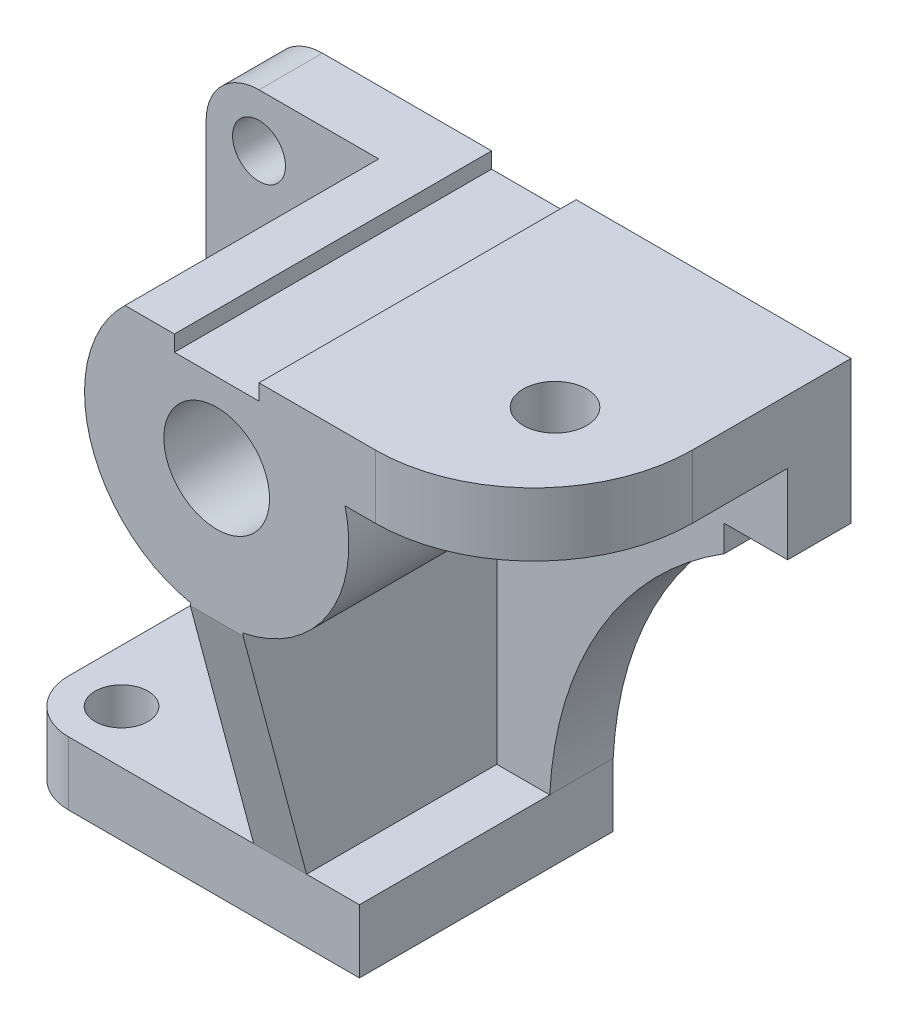
ISO-10303-21;
HEADER;
FILE_DESCRIPTION(('STEP AP214'),'2;1');
FILE_NAME('part.step','',(''),(''),'','','');
FILE_SCHEMA(('AUTOMOTIVE_DESIGN { 1 0 10303 214 1 1 1 1 }'));
ENDSEC;
DATA;
#1=APPLICATION_CONTEXT('core data for automotive mechanical design processes');
#2=APPLICATION_PROTOCOL_DEFINITION('international standard','automotive_design',2000,#1);
#3=PRODUCT_CONTEXT('',#1,'mechanical');
#4=PRODUCT('Part','Part','',(#3));
#5=PRODUCT_RELATED_PRODUCT_CATEGORY('part','',(#4));
#6=PRODUCT_DEFINITION_FORMATION('','',#4);
#7=PRODUCT_DEFINITION_CONTEXT('part definition',#1,'design');
#8=PRODUCT_DEFINITION('design','',#6,#7);
#9=PRODUCT_DEFINITION_SHAPE('','',#8);
#10=(LENGTH_UNIT() NAMED_UNIT(*) SI_UNIT(.MILLI.,.METRE.));
#11=(NAMED_UNIT(*) PLANE_ANGLE_UNIT() SI_UNIT($,.RADIAN.));
#12=(NAMED_UNIT(*) SI_UNIT($,.STERADIAN.) SOLID_ANGLE_UNIT());
#13=UNCERTAINTY_MEASURE_WITH_UNIT(LENGTH_MEASURE(1.E-05),#10,'distance_accuracy_value','');
#14=(GEOMETRIC_REPRESENTATION_CONTEXT(3) GLOBAL_UNCERTAINTY_ASSIGNED_CONTEXT((#13)) GLOBAL_UNIT_ASSIGNED_CONTEXT((#10,
#11,#12)) REPRESENTATION_CONTEXT('',''));
#15=CARTESIAN_POINT('',(0.,0.,0.));
#16=DIRECTION('',(0.,0.,1.));
#17=DIRECTION('',(1.,0.,0.));
#18=AXIS2_PLACEMENT_3D('',#15,#16,#17);
#19=CARTESIAN_POINT('',(102.413647614437,8.52410051292082,-12.));
#20=DIRECTION('',(0.,0.,1.));
#21=DIRECTION('',(1.,0.,0.));
#22=AXIS2_PLACEMENT_3D('',#19,#20,#21);
#23=PLANE('',#22);
#24=CARTESIAN_POINT('',(-22.5,90.,-12.));
#25=DIRECTION('',(0.,0.,1.));
#26=DIRECTION('',(1.,0.,0.));
#27=AXIS2_PLACEMENT_3D('',#24,#25,#26);
#28=CIRCLE('',#27,5.);
#29=CARTESIAN_POINT('',(-17.5,90.,-12.));
#30=VERTEX_POINT('',#29);
#31=EDGE_CURVE('E776',#30,#30,#28,.T.);
#32=ORIENTED_EDGE('',*,*,#31,.F.);
#33=EDGE_LOOP('',(#32));
#34=FACE_BOUND('',#33,.T.);
#35=DIRECTION('',(-1.,0.,0.));
#36=VECTOR('',#35,1.);
#37=CARTESIAN_POINT('',(32.5,12.,-12.));
#38=LINE('',#37,#36);
#39=CARTESIAN_POINT('',(12.5,12.,-12.));
#40=VERTEX_POINT('',#39);
#41=CARTESIAN_POINT('',(-32.5,12.,-12.));
#42=VERTEX_POINT('',#41);
#43=EDGE_CURVE('E300',#40,#42,#38,.T.);
#44=ORIENTED_EDGE('',*,*,#43,.F.);
#45=DIRECTION('',(0.,1.,0.));
#46=VECTOR('',#45,1.);
#47=CARTESIAN_POINT('',(12.5,8.52410051292082,-12.));
#48=LINE('',#47,#46);
#49=CARTESIAN_POINT('',(12.5,57.5051025721682,-12.));
#50=VERTEX_POINT('',#49);
#51=EDGE_CURVE('E232',#40,#50,#48,.T.);
#52=ORIENTED_EDGE('',*,*,#51,.T.);
#53=CARTESIAN_POINT('',(17.5,82.,-12.));
#54=DIRECTION('',(0.,0.,1.));
#55=DIRECTION('',(1.,0.,0.));
#56=AXIS2_PLACEMENT_3D('',#53,#54,#55);
#57=CIRCLE('',#56,25.);
#58=CARTESIAN_POINT('',(0.15064842710252,100.,-12.));
#59=VERTEX_POINT('',#58);
#60=EDGE_CURVE('E289',#59,#50,#57,.T.);
#61=ORIENTED_EDGE('',*,*,#60,.F.);
#62=DIRECTION('',(1.,0.,0.));
#63=VECTOR('',#62,1.);
#64=CARTESIAN_POINT('',(-32.5,100.,-12.));
#65=LINE('',#64,#63);
#66=CARTESIAN_POINT('',(-22.5,100.,-12.));
#67=VERTEX_POINT('',#66);
#68=EDGE_CURVE('E297',#67,#59,#65,.T.);
#69=ORIENTED_EDGE('',*,*,#68,.F.);
#70=CARTESIAN_POINT('',(-22.5,90.,-12.));
#71=DIRECTION('',(0.,0.,1.));
#72=DIRECTION('',(1.,0.,0.));
#73=AXIS2_PLACEMENT_3D('',#70,#71,#72);
#74=CIRCLE('',#73,10.);
#75=CARTESIAN_POINT('',(-32.5,90.,-12.));
#76=VERTEX_POINT('',#75);
#77=EDGE_CURVE('E381',#67,#76,#74,.T.);
#78=ORIENTED_EDGE('',*,*,#77,.T.);
#79=DIRECTION('',(0.,1.,0.));
#80=VECTOR('',#79,1.);
#81=CARTESIAN_POINT('',(-32.5,12.,-12.));
#82=LINE('',#81,#80);
#83=EDGE_CURVE('E298',#42,#76,#82,.T.);
#84=ORIENTED_EDGE('',*,*,#83,.F.);
#85=EDGE_LOOP('',(#44,#52,#61,#69,#78,#84));
#86=FACE_BOUND('',#85,.T.);
#87=ADVANCED_FACE('F43',(#34,#86),#23,.T.);
#88=CARTESIAN_POINT('',(0.,12.,0.));
#89=DIRECTION('',(0.,-1.,0.));
#90=DIRECTION('',(0.,0.,-1.));
#91=AXIS2_PLACEMENT_3D('',#88,#89,#90);
#92=PLANE('',#91);
#93=CARTESIAN_POINT('',(-22.5,12.,14.));
#94=DIRECTION('',(0.,1.,0.));
#95=DIRECTION('',(0.,0.,1.));
#96=AXIS2_PLACEMENT_3D('',#93,#94,#95);
#97=CIRCLE('',#96,5.);
#98=CARTESIAN_POINT('',(-22.5,12.,19.));
#99=VERTEX_POINT('',#98);
#100=EDGE_CURVE('E783',#99,#99,#97,.T.);
#101=ORIENTED_EDGE('',*,*,#100,.F.);
#102=EDGE_LOOP('',(#101));
#103=FACE_BOUND('',#102,.T.);
#104=DIRECTION('',(0.,0.,1.));
#105=VECTOR('',#104,1.);
#106=CARTESIAN_POINT('',(12.5,12.,0.));
#107=LINE('',#106,#105);
#108=CARTESIAN_POINT('',(12.5,12.,24.));
#109=VERTEX_POINT('',#108);
#110=EDGE_CURVE('E238',#40,#109,#107,.T.);
#111=ORIENTED_EDGE('',*,*,#110,.F.);
#112=ORIENTED_EDGE('',*,*,#43,.T.);
#113=DIRECTION('',(0.,0.,1.));
#114=VECTOR('',#113,1.);
#115=CARTESIAN_POINT('',(-32.5,12.,24.));
#116=LINE('',#115,#114);
#117=CARTESIAN_POINT('',(-32.5,12.,14.));
#118=VERTEX_POINT('',#117);
#119=EDGE_CURVE('E344',#42,#118,#116,.T.);
#120=ORIENTED_EDGE('',*,*,#119,.T.);
#121=CARTESIAN_POINT('',(-22.5,12.,14.));
#122=DIRECTION('',(0.,-1.,0.));
#123=DIRECTION('',(0.,0.,-1.));
#124=AXIS2_PLACEMENT_3D('',#121,#122,#123);
#125=CIRCLE('',#124,10.);
#126=CARTESIAN_POINT('',(-22.5,12.,24.));
#127=VERTEX_POINT('',#126);
#128=EDGE_CURVE('E374',#118,#127,#125,.F.);
#129=ORIENTED_EDGE('',*,*,#128,.T.);
#130=DIRECTION('',(1.,0.,0.));
#131=VECTOR('',#130,1.);
#132=CARTESIAN_POINT('',(-32.5,12.,24.));
#133=LINE('',#132,#131);
#134=EDGE_CURVE('E350',#127,#109,#133,.T.);
#135=ORIENTED_EDGE('',*,*,#134,.T.);
#136=EDGE_LOOP('',(#111,#112,#120,#129,#135));
#137=FACE_BOUND('',#136,.T.);
#138=ADVANCED_FACE('F472',(#103,#137),#92,.F.);
#139=CARTESIAN_POINT('',(17.5,82.,36.));
#140=DIRECTION('',(0.,0.,-1.));
#141=DIRECTION('',(-1.,0.,0.));
#142=AXIS2_PLACEMENT_3D('',#139,#140,#141);
#143=CYLINDRICAL_SURFACE('',#142,25.);
#144=DIRECTION('',(0.,0.,-1.));
#145=VECTOR('',#144,1.);
#146=CARTESIAN_POINT('',(12.5,57.5051025721682,36.));
#147=LINE('',#146,#145);
#148=CARTESIAN_POINT('',(12.5,57.5051025721682,36.));
#149=VERTEX_POINT('',#148);
#150=EDGE_CURVE('E214',#149,#50,#147,.T.);
#151=ORIENTED_EDGE('',*,*,#150,.F.);
#152=CARTESIAN_POINT('',(17.5,82.,36.));
#153=DIRECTION('',(0.,0.,1.));
#154=DIRECTION('',(1.,0.,0.));
#155=AXIS2_PLACEMENT_3D('',#152,#153,#154);
#156=CIRCLE('',#155,25.);
#157=CARTESIAN_POINT('',(0.15064842710252,100.,36.));
#158=VERTEX_POINT('',#157);
#159=EDGE_CURVE('E282',#158,#149,#156,.T.);
#160=ORIENTED_EDGE('',*,*,#159,.F.);
#161=DIRECTION('',(0.,0.,-1.));
#162=VECTOR('',#161,1.);
#163=CARTESIAN_POINT('',(0.15064842710252,100.,36.));
#164=LINE('',#163,#162);
#165=EDGE_CURVE('E287',#158,#59,#164,.T.);
#166=ORIENTED_EDGE('',*,*,#165,.T.);
#167=ORIENTED_EDGE('',*,*,#60,.T.);
#168=EDGE_LOOP('',(#151,#160,#166,#167));
#169=FACE_BOUND('',#168,.T.);
#170=ADVANCED_FACE('F458',(#169),#143,.T.);
#171=CARTESIAN_POINT('',(-32.5,100.,-12.));
#172=DIRECTION('',(0.,1.,0.));
#173=DIRECTION('',(-1.,0.,0.));
#174=AXIS2_PLACEMENT_3D('',#171,#172,#173);
#175=PLANE('',#174);
#176=CARTESIAN_POINT('',(57.5,100.,12.));
#177=DIRECTION('',(0.,1.,0.));
#178=DIRECTION('',(-1.,0.,0.));
#179=AXIS2_PLACEMENT_3D('',#176,#177,#178);
#180=CIRCLE('',#179,5.99999999999999);
#181=CARTESIAN_POINT('',(51.5,100.,12.));
#182=VERTEX_POINT('',#181);
#183=EDGE_CURVE('E771',#182,#182,#180,.T.);
#184=ORIENTED_EDGE('',*,*,#183,.F.);
#185=EDGE_LOOP('',(#184));
#186=FACE_BOUND('',#185,.T.);
#187=DIRECTION('',(-1.,0.,0.));
#188=VECTOR('',#187,1.);
#189=CARTESIAN_POINT('',(0.15064842710252,100.,36.));
#190=LINE('',#189,#188);
#191=CARTESIAN_POINT('',(47.5,100.,36.));
#192=VERTEX_POINT('',#191);
#193=CARTESIAN_POINT('',(25.5,100.,36.));
#194=VERTEX_POINT('',#193);
#195=EDGE_CURVE('E283',#192,#194,#190,.T.);
#196=ORIENTED_EDGE('',*,*,#195,.F.);
#197=CARTESIAN_POINT('',(47.5,100.,6.));
#198=DIRECTION('',(0.,1.,0.));
#199=DIRECTION('',(-1.,0.,0.));
#200=AXIS2_PLACEMENT_3D('',#197,#198,#199);
#201=CIRCLE('',#200,30.);
#202=CARTESIAN_POINT('',(77.5,100.,6.));
#203=VERTEX_POINT('',#202);
#204=EDGE_CURVE('E392',#192,#203,#201,.T.);
#205=ORIENTED_EDGE('',*,*,#204,.T.);
#206=DIRECTION('',(0.,0.,-1.));
#207=VECTOR('',#206,1.);
#208=CARTESIAN_POINT('',(77.5,100.,-12.));
#209=LINE('',#208,#207);
#210=CARTESIAN_POINT('',(77.5,100.,-24.));
#211=VERTEX_POINT('',#210);
#212=EDGE_CURVE('E313',#203,#211,#209,.T.);
#213=ORIENTED_EDGE('',*,*,#212,.T.);
#214=DIRECTION('',(1.,0.,0.));
#215=VECTOR('',#214,1.);
#216=CARTESIAN_POINT('',(-32.5,100.,-24.));
#217=LINE('',#216,#215);
#218=CARTESIAN_POINT('',(25.5,100.,-24.));
#219=VERTEX_POINT('',#218);
#220=EDGE_CURVE('E292',#219,#211,#217,.T.);
#221=ORIENTED_EDGE('',*,*,#220,.F.);
#222=DIRECTION('',(0.,0.,-1.));
#223=VECTOR('',#222,1.);
#224=CARTESIAN_POINT('',(25.5,100.,-12.));
#225=LINE('',#224,#223);
#226=EDGE_CURVE('E279',#194,#219,#225,.T.);
#227=ORIENTED_EDGE('',*,*,#226,.F.);
#228=EDGE_LOOP('',(#196,#205,#213,#221,#227));
#229=FACE_BOUND('',#228,.T.);
#230=ADVANCED_FACE('F391',(#186,#229),#175,.T.);
#231=DIRECTION('',(0.,1.,0.));
#232=VECTOR('',#231,1.);
#233=CARTESIAN_POINT('',(22.5,8.52410051292082,-12.));
#234=LINE('',#233,#232);
#235=CARTESIAN_POINT('',(22.5,12.,-12.));
#236=VERTEX_POINT('',#235);
#237=CARTESIAN_POINT('',(22.5,57.5051025721682,-12.));
#238=VERTEX_POINT('',#237);
#239=EDGE_CURVE('E241',#236,#238,#234,.T.);
#240=ORIENTED_EDGE('',*,*,#239,.F.);
#241=CARTESIAN_POINT('',(32.5,12.,-12.));
#242=VERTEX_POINT('',#241);
#243=EDGE_CURVE('E291',#242,#236,#38,.T.);
#244=ORIENTED_EDGE('',*,*,#243,.F.);
#245=CARTESIAN_POINT('',(102.413647614437,8.52410051292082,-12.));
#246=DIRECTION('',(0.,0.,1.));
#247=DIRECTION('',(1.,0.,0.));
#248=AXIS2_PLACEMENT_3D('',#245,#246,#247);
#249=CIRCLE('',#248,70.);
#250=CARTESIAN_POINT('',(65.5,68.,-12.));
#251=VERTEX_POINT('',#250);
#252=EDGE_CURVE('E311',#251,#242,#249,.T.);
#253=ORIENTED_EDGE('',*,*,#252,.F.);
#254=DIRECTION('',(0.,-1.,0.));
#255=VECTOR('',#254,1.);
#256=CARTESIAN_POINT('',(65.5,73.,-12.));
#257=LINE('',#256,#255);
#258=CARTESIAN_POINT('',(65.5,73.,-12.));
#259=VERTEX_POINT('',#258);
#260=EDGE_CURVE('E308',#259,#251,#257,.T.);
#261=ORIENTED_EDGE('',*,*,#260,.F.);
#262=DIRECTION('',(-1.,0.,0.));
#263=VECTOR('',#262,1.);
#264=CARTESIAN_POINT('',(77.5,73.,-12.));
#265=LINE('',#264,#263);
#266=CARTESIAN_POINT('',(77.5,73.,-12.));
#267=VERTEX_POINT('',#266);
#268=EDGE_CURVE('E304',#267,#259,#265,.T.);
#269=ORIENTED_EDGE('',*,*,#268,.F.);
#270=DIRECTION('',(0.,-1.,0.));
#271=VECTOR('',#270,1.);
#272=CARTESIAN_POINT('',(77.5,100.,-12.));
#273=LINE('',#272,#271);
#274=CARTESIAN_POINT('',(77.5,88.,-12.));
#275=VERTEX_POINT('',#274);
#276=EDGE_CURVE('E303',#275,#267,#273,.T.);
#277=ORIENTED_EDGE('',*,*,#276,.F.);
#278=DIRECTION('',(1.,0.,0.));
#279=VECTOR('',#278,1.);
#280=CARTESIAN_POINT('',(102.413647614437,88.,-12.));
#281=LINE('',#280,#279);
#282=CARTESIAN_POINT('',(41.7693221990232,88.,-12.));
#283=VERTEX_POINT('',#282);
#284=EDGE_CURVE('E251',#283,#275,#281,.T.);
#285=ORIENTED_EDGE('',*,*,#284,.F.);
#286=EDGE_CURVE('E278',#238,#283,#57,.T.);
#287=ORIENTED_EDGE('',*,*,#286,.F.);
#288=EDGE_LOOP('',(#240,#244,#253,#261,#269,#277,#285,#287));
#289=FACE_BOUND('',#288,.T.);
#290=ADVANCED_FACE('F411',(#289),#23,.T.);
#291=CARTESIAN_POINT('',(32.5,12.,24.));
#292=DIRECTION('',(-1.,0.,0.));
#293=DIRECTION('',(0.,0.,1.));
#294=AXIS2_PLACEMENT_3D('',#291,#292,#293);
#295=PLANE('',#294);
#296=DIRECTION('',(0.,0.,-1.));
#297=VECTOR('',#296,1.);
#298=CARTESIAN_POINT('',(32.5,0.,24.));
#299=LINE('',#298,#297);
#300=CARTESIAN_POINT('',(32.5,0.,24.));
#301=VERTEX_POINT('',#300);
#302=CARTESIAN_POINT('',(32.5,0.,-24.));
#303=VERTEX_POINT('',#302);
#304=EDGE_CURVE('E331',#301,#303,#299,.T.);
#305=ORIENTED_EDGE('',*,*,#304,.T.);
#306=DIRECTION('',(0.,-1.,0.));
#307=VECTOR('',#306,1.);
#308=CARTESIAN_POINT('',(32.5,12.,-24.));
#309=LINE('',#308,#307);
#310=CARTESIAN_POINT('',(32.5,12.,-24.));
#311=VERTEX_POINT('',#310);
#312=EDGE_CURVE('E364',#311,#303,#309,.T.);
#313=ORIENTED_EDGE('',*,*,#312,.F.);
#314=DIRECTION('',(0.,0.,-1.));
#315=VECTOR('',#314,1.);
#316=CARTESIAN_POINT('',(32.5,12.,-12.));
#317=LINE('',#316,#315);
#318=EDGE_CURVE('E326',#242,#311,#317,.T.);
#319=ORIENTED_EDGE('',*,*,#318,.F.);
#320=DIRECTION('',(0.,0.,-1.));
#321=VECTOR('',#320,1.);
#322=CARTESIAN_POINT('',(32.5,12.,24.));
#323=LINE('',#322,#321);
#324=CARTESIAN_POINT('',(32.5,12.,24.));
#325=VERTEX_POINT('',#324);
#326=EDGE_CURVE('E338',#325,#242,#323,.T.);
#327=ORIENTED_EDGE('',*,*,#326,.F.);
#328=DIRECTION('',(0.,-1.,0.));
#329=VECTOR('',#328,1.);
#330=CARTESIAN_POINT('',(32.5,12.,24.));
#331=LINE('',#330,#329);
#332=EDGE_CURVE('E348',#325,#301,#331,.T.);
#333=ORIENTED_EDGE('',*,*,#332,.T.);
#334=EDGE_LOOP('',(#305,#313,#319,#327,#333));
#335=FACE_BOUND('',#334,.T.);
#336=ADVANCED_FACE('F482',(#335),#295,.F.);
#337=CARTESIAN_POINT('',(-32.5,12.,-24.));
#338=DIRECTION('',(0.,0.,1.));
#339=DIRECTION('',(1.,0.,0.));
#340=AXIS2_PLACEMENT_3D('',#337,#338,#339);
#341=PLANE('',#340);
#342=CARTESIAN_POINT('',(17.5,82.,-24.));
#343=DIRECTION('',(0.,0.,1.));
#344=DIRECTION('',(1.,0.,0.));
#345=AXIS2_PLACEMENT_3D('',#342,#343,#344);
#346=CIRCLE('',#345,10.);
#347=CARTESIAN_POINT('',(27.5,82.,-24.));
#348=VERTEX_POINT('',#347);
#349=EDGE_CURVE('E789',#348,#348,#346,.F.);
#350=ORIENTED_EDGE('',*,*,#349,.F.);
#351=EDGE_LOOP('',(#350));
#352=FACE_BOUND('',#351,.T.);
#353=CARTESIAN_POINT('',(-22.5,90.,-24.));
#354=DIRECTION('',(0.,0.,1.));
#355=DIRECTION('',(1.,0.,0.));
#356=AXIS2_PLACEMENT_3D('',#353,#354,#355);
#357=CIRCLE('',#356,5.);
#358=CARTESIAN_POINT('',(-17.5,90.,-24.));
#359=VERTEX_POINT('',#358);
#360=EDGE_CURVE('E780',#359,#359,#357,.T.);
#361=ORIENTED_EDGE('',*,*,#360,.T.);
#362=EDGE_LOOP('',(#361));
#363=FACE_BOUND('',#362,.T.);
#364=DIRECTION('',(-1.,0.,0.));
#365=VECTOR('',#364,1.);
#366=CARTESIAN_POINT('',(-32.5,0.,-24.));
#367=LINE('',#366,#365);
#368=CARTESIAN_POINT('',(-32.5,0.,-24.));
#369=VERTEX_POINT('',#368);
#370=EDGE_CURVE('E354',#303,#369,#367,.T.);
#371=ORIENTED_EDGE('',*,*,#370,.T.);
#372=DIRECTION('',(0.,-1.,0.));
#373=VECTOR('',#372,1.);
#374=CARTESIAN_POINT('',(-32.5,12.,-24.));
#375=LINE('',#374,#373);
#376=CARTESIAN_POINT('',(-32.5,90.,-24.));
#377=VERTEX_POINT('',#376);
#378=EDGE_CURVE('E363',#377,#369,#375,.T.);
#379=ORIENTED_EDGE('',*,*,#378,.F.);
#380=CARTESIAN_POINT('',(-22.5,90.,-24.));
#381=DIRECTION('',(0.,0.,1.));
#382=DIRECTION('',(1.,0.,0.));
#383=AXIS2_PLACEMENT_3D('',#380,#381,#382);
#384=CIRCLE('',#383,10.);
#385=CARTESIAN_POINT('',(-22.5,100.,-24.));
#386=VERTEX_POINT('',#385);
#387=EDGE_CURVE('E379',#377,#386,#384,.F.);
#388=ORIENTED_EDGE('',*,*,#387,.T.);
#389=CARTESIAN_POINT('',(9.50000000000002,100.,-24.));
#390=VERTEX_POINT('',#389);
#391=EDGE_CURVE('E314',#386,#390,#217,.T.);
#392=ORIENTED_EDGE('',*,*,#391,.T.);
#393=DIRECTION('',(0.,-1.,0.));
#394=VECTOR('',#393,1.);
#395=CARTESIAN_POINT('',(9.50000000000002,97.,-24.));
#396=LINE('',#395,#394);
#397=CARTESIAN_POINT('',(9.50000000000002,97.,-24.));
#398=VERTEX_POINT('',#397);
#399=EDGE_CURVE('E262',#390,#398,#396,.T.);
#400=ORIENTED_EDGE('',*,*,#399,.T.);
#401=DIRECTION('',(1.,0.,0.));
#402=VECTOR('',#401,1.);
#403=CARTESIAN_POINT('',(9.50000000000002,97.,-24.));
#404=LINE('',#403,#402);
#405=CARTESIAN_POINT('',(25.5,97.,-24.));
#406=VERTEX_POINT('',#405);
#407=EDGE_CURVE('E263',#398,#406,#404,.T.);
#408=ORIENTED_EDGE('',*,*,#407,.T.);
#409=DIRECTION('',(0.,1.,0.));
#410=VECTOR('',#409,1.);
#411=CARTESIAN_POINT('',(25.5,97.,-24.));
#412=LINE('',#411,#410);
#413=EDGE_CURVE('E259',#406,#219,#412,.T.);
#414=ORIENTED_EDGE('',*,*,#413,.T.);
#415=ORIENTED_EDGE('',*,*,#220,.T.);
#416=DIRECTION('',(0.,-1.,0.));
#417=VECTOR('',#416,1.);
#418=CARTESIAN_POINT('',(77.5,100.,-24.));
#419=LINE('',#418,#417);
#420=CARTESIAN_POINT('',(77.5,73.,-24.));
#421=VERTEX_POINT('',#420);
#422=EDGE_CURVE('E319',#211,#421,#419,.T.);
#423=ORIENTED_EDGE('',*,*,#422,.T.);
#424=DIRECTION('',(-1.,0.,0.));
#425=VECTOR('',#424,1.);
#426=CARTESIAN_POINT('',(77.5,73.,-24.));
#427=LINE('',#426,#425);
#428=CARTESIAN_POINT('',(65.5,73.,-24.));
#429=VERTEX_POINT('',#428);
#430=EDGE_CURVE('E318',#421,#429,#427,.T.);
#431=ORIENTED_EDGE('',*,*,#430,.T.);
#432=DIRECTION('',(0.,-1.,0.));
#433=VECTOR('',#432,1.);
#434=CARTESIAN_POINT('',(65.5,73.,-24.));
#435=LINE('',#434,#433);
#436=CARTESIAN_POINT('',(65.5,68.,-24.));
#437=VERTEX_POINT('',#436);
#438=EDGE_CURVE('E324',#429,#437,#435,.T.);
#439=ORIENTED_EDGE('',*,*,#438,.T.);
#440=CARTESIAN_POINT('',(102.413647614437,8.52410051292082,-24.));
#441=DIRECTION('',(0.,0.,1.));
#442=DIRECTION('',(1.,0.,0.));
#443=AXIS2_PLACEMENT_3D('',#440,#441,#442);
#444=CIRCLE('',#443,70.);
#445=EDGE_CURVE('E327',#437,#311,#444,.T.);
#446=ORIENTED_EDGE('',*,*,#445,.T.);
#447=ORIENTED_EDGE('',*,*,#312,.T.);
#448=EDGE_LOOP('',(#371,#379,#388,#392,#400,#408,#414,#415,#423,#431,#439,#446,#447));
#449=FACE_BOUND('',#448,.T.);
#450=ADVANCED_FACE('F421',(#352,#363,#449),#341,.F.);
#451=CARTESIAN_POINT('',(-32.5,12.,24.));
#452=DIRECTION('',(1.,0.,0.));
#453=DIRECTION('',(0.,0.,-1.));
#454=AXIS2_PLACEMENT_3D('',#451,#452,#453);
#455=PLANE('',#454);
#456=ORIENTED_EDGE('',*,*,#83,.T.);
#457=DIRECTION('',(0.,0.,-1.));
#458=VECTOR('',#457,1.);
#459=CARTESIAN_POINT('',(-32.5,90.,-24.));
#460=LINE('',#459,#458);
#461=EDGE_CURVE('E380',#76,#377,#460,.T.);
#462=ORIENTED_EDGE('',*,*,#461,.T.);
#463=ORIENTED_EDGE('',*,*,#378,.T.);
#464=DIRECTION('',(0.,0.,1.));
#465=VECTOR('',#464,1.);
#466=CARTESIAN_POINT('',(-32.5,0.,24.));
#467=LINE('',#466,#465);
#468=CARTESIAN_POINT('',(-32.5,0.,14.));
#469=VERTEX_POINT('',#468);
#470=EDGE_CURVE('E355',#369,#469,#467,.T.);
#471=ORIENTED_EDGE('',*,*,#470,.T.);
#472=DIRECTION('',(0.,-1.,0.));
#473=VECTOR('',#472,1.);
#474=CARTESIAN_POINT('',(-32.5,12.,14.));
#475=LINE('',#474,#473);
#476=EDGE_CURVE('E375',#469,#118,#475,.F.);
#477=ORIENTED_EDGE('',*,*,#476,.T.);
#478=ORIENTED_EDGE('',*,*,#119,.F.);
#479=EDGE_LOOP('',(#456,#462,#463,#471,#477,#478));
#480=FACE_BOUND('',#479,.T.);
#481=ADVANCED_FACE('F446',(#480),#455,.F.);
#482=CARTESIAN_POINT('',(-32.5,12.,24.));
#483=DIRECTION('',(0.,0.,-1.));
#484=DIRECTION('',(-1.,0.,0.));
#485=AXIS2_PLACEMENT_3D('',#482,#483,#484);
#486=PLANE('',#485);
#487=ORIENTED_EDGE('',*,*,#134,.F.);
#488=DIRECTION('',(0.,-1.,0.));
#489=VECTOR('',#488,1.);
#490=CARTESIAN_POINT('',(-22.5,12.,24.));
#491=LINE('',#490,#489);
#492=CARTESIAN_POINT('',(-22.5,0.,24.));
#493=VERTEX_POINT('',#492);
#494=EDGE_CURVE('E370',#127,#493,#491,.T.);
#495=ORIENTED_EDGE('',*,*,#494,.T.);
#496=DIRECTION('',(1.,0.,0.));
#497=VECTOR('',#496,1.);
#498=CARTESIAN_POINT('',(-32.5,0.,24.));
#499=LINE('',#498,#497);
#500=EDGE_CURVE('E341',#493,#301,#499,.T.);
#501=ORIENTED_EDGE('',*,*,#500,.T.);
#502=ORIENTED_EDGE('',*,*,#332,.F.);
#503=CARTESIAN_POINT('',(22.5,12.,24.));
#504=VERTEX_POINT('',#503);
#505=EDGE_CURVE('E347',#504,#325,#133,.T.);
#506=ORIENTED_EDGE('',*,*,#505,.F.);
#507=DIRECTION('',(-1.,0.,0.));
#508=VECTOR('',#507,1.);
#509=CARTESIAN_POINT('',(0.,12.,24.));
#510=LINE('',#509,#508);
#511=EDGE_CURVE('E227',#504,#109,#510,.T.);
#512=ORIENTED_EDGE('',*,*,#511,.T.);
#513=EDGE_LOOP('',(#487,#495,#501,#502,#506,#512));
#514=FACE_BOUND('',#513,.T.);
#515=ADVANCED_FACE('F470',(#514),#486,.F.);
#516=ORIENTED_EDGE('',*,*,#243,.T.);
#517=DIRECTION('',(0.,0.,1.));
#518=VECTOR('',#517,1.);
#519=CARTESIAN_POINT('',(22.5,12.,0.));
#520=LINE('',#519,#518);
#521=EDGE_CURVE('E243',#236,#504,#520,.T.);
#522=ORIENTED_EDGE('',*,*,#521,.T.);
#523=ORIENTED_EDGE('',*,*,#505,.T.);
#524=ORIENTED_EDGE('',*,*,#326,.T.);
#525=EDGE_LOOP('',(#516,#522,#523,#524));
#526=FACE_BOUND('',#525,.T.);
#527=ADVANCED_FACE('F488',(#526),#92,.F.);
#528=CARTESIAN_POINT('',(0.,0.,0.));
#529=DIRECTION('',(0.,-1.,0.));
#530=DIRECTION('',(0.,0.,-1.));
#531=AXIS2_PLACEMENT_3D('',#528,#529,#530);
#532=PLANE('',#531);
#533=CARTESIAN_POINT('',(-22.5,0.,14.));
#534=DIRECTION('',(0.,1.,0.));
#535=DIRECTION('',(0.,0.,1.));
#536=AXIS2_PLACEMENT_3D('',#533,#534,#535);
#537=CIRCLE('',#536,5.);
#538=CARTESIAN_POINT('',(-22.5,0.,19.));
#539=VERTEX_POINT('',#538);
#540=EDGE_CURVE('E785',#539,#539,#537,.T.);
#541=ORIENTED_EDGE('',*,*,#540,.T.);
#542=EDGE_LOOP('',(#541));
#543=FACE_BOUND('',#542,.T.);
#544=ORIENTED_EDGE('',*,*,#470,.F.);
#545=ORIENTED_EDGE('',*,*,#370,.F.);
#546=ORIENTED_EDGE('',*,*,#304,.F.);
#547=ORIENTED_EDGE('',*,*,#500,.F.);
#548=CARTESIAN_POINT('',(-22.5,0.,14.));
#549=DIRECTION('',(0.,-1.,0.));
#550=DIRECTION('',(0.,0.,-1.));
#551=AXIS2_PLACEMENT_3D('',#548,#549,#550);
#552=CIRCLE('',#551,10.);
#553=EDGE_CURVE('E369',#493,#469,#552,.T.);
#554=ORIENTED_EDGE('',*,*,#553,.T.);
#555=EDGE_LOOP('',(#544,#545,#546,#547,#554));
#556=FACE_BOUND('',#555,.T.);
#557=ADVANCED_FACE('F476',(#543,#556),#532,.T.);
#558=CARTESIAN_POINT('',(-22.5,12.,14.));
#559=DIRECTION('',(0.,-1.,0.));
#560=DIRECTION('',(0.,0.,-1.));
#561=AXIS2_PLACEMENT_3D('',#558,#559,#560);
#562=CYLINDRICAL_SURFACE('',#561,10.);
#563=ORIENTED_EDGE('',*,*,#128,.F.);
#564=ORIENTED_EDGE('',*,*,#476,.F.);
#565=ORIENTED_EDGE('',*,*,#553,.F.);
#566=ORIENTED_EDGE('',*,*,#494,.F.);
#567=EDGE_LOOP('',(#563,#564,#565,#566));
#568=FACE_BOUND('',#567,.T.);
#569=ADVANCED_FACE('F473',(#568),#562,.T.);
#570=CARTESIAN_POINT('',(102.413647614437,8.52410051292082,-12.));
#571=DIRECTION('',(0.,0.,-1.));
#572=DIRECTION('',(-1.,0.,0.));
#573=AXIS2_PLACEMENT_3D('',#570,#571,#572);
#574=CYLINDRICAL_SURFACE('',#573,70.);
#575=ORIENTED_EDGE('',*,*,#445,.F.);
#576=DIRECTION('',(0.,0.,-1.));
#577=VECTOR('',#576,1.);
#578=CARTESIAN_POINT('',(65.5,68.,-12.));
#579=LINE('',#578,#577);
#580=EDGE_CURVE('E332',#251,#437,#579,.T.);
#581=ORIENTED_EDGE('',*,*,#580,.F.);
#582=ORIENTED_EDGE('',*,*,#252,.T.);
#583=ORIENTED_EDGE('',*,*,#318,.T.);
#584=EDGE_LOOP('',(#575,#581,#582,#583));
#585=FACE_BOUND('',#584,.T.);
#586=ADVANCED_FACE('F490',(#585),#574,.F.);
#587=CARTESIAN_POINT('',(65.5,73.,-12.));
#588=DIRECTION('',(1.,0.,0.));
#589=DIRECTION('',(0.,1.,0.));
#590=AXIS2_PLACEMENT_3D('',#587,#588,#589);
#591=PLANE('',#590);
#592=ORIENTED_EDGE('',*,*,#438,.F.);
#593=DIRECTION('',(0.,0.,-1.));
#594=VECTOR('',#593,1.);
#595=CARTESIAN_POINT('',(65.5,73.,-12.));
#596=LINE('',#595,#594);
#597=EDGE_CURVE('E333',#259,#429,#596,.T.);
#598=ORIENTED_EDGE('',*,*,#597,.F.);
#599=ORIENTED_EDGE('',*,*,#260,.T.);
#600=ORIENTED_EDGE('',*,*,#580,.T.);
#601=EDGE_LOOP('',(#592,#598,#599,#600));
#602=FACE_BOUND('',#601,.T.);
#603=ADVANCED_FACE('F493',(#602),#591,.T.);
#604=CARTESIAN_POINT('',(77.5,73.,-12.));
#605=DIRECTION('',(0.,-1.,0.));
#606=DIRECTION('',(0.,0.,-1.));
#607=AXIS2_PLACEMENT_3D('',#604,#605,#606);
#608=PLANE('',#607);
#609=ORIENTED_EDGE('',*,*,#430,.F.);
#610=DIRECTION('',(0.,0.,-1.));
#611=VECTOR('',#610,1.);
#612=CARTESIAN_POINT('',(77.5,73.,-12.));
#613=LINE('',#612,#611);
#614=EDGE_CURVE('E337',#267,#421,#613,.T.);
#615=ORIENTED_EDGE('',*,*,#614,.F.);
#616=ORIENTED_EDGE('',*,*,#268,.T.);
#617=ORIENTED_EDGE('',*,*,#597,.T.);
#618=EDGE_LOOP('',(#609,#615,#616,#617));
#619=FACE_BOUND('',#618,.T.);
#620=ADVANCED_FACE('F420',(#619),#608,.T.);
#621=CARTESIAN_POINT('',(77.5,100.,-12.));
#622=DIRECTION('',(1.,0.,0.));
#623=DIRECTION('',(0.,0.,-1.));
#624=AXIS2_PLACEMENT_3D('',#621,#622,#623);
#625=PLANE('',#624);
#626=ORIENTED_EDGE('',*,*,#212,.F.);
#627=DIRECTION('',(0.,1.,0.));
#628=VECTOR('',#627,1.);
#629=CARTESIAN_POINT('',(77.5,100.,6.));
#630=LINE('',#629,#628);
#631=CARTESIAN_POINT('',(77.5,88.,6.));
#632=VERTEX_POINT('',#631);
#633=EDGE_CURVE('E51',#203,#632,#630,.F.);
#634=ORIENTED_EDGE('',*,*,#633,.T.);
#635=DIRECTION('',(0.,0.,-1.));
#636=VECTOR('',#635,1.);
#637=CARTESIAN_POINT('',(77.5,88.,-24.));
#638=LINE('',#637,#636);
#639=EDGE_CURVE('E246',#632,#275,#638,.T.);
#640=ORIENTED_EDGE('',*,*,#639,.T.);
#641=ORIENTED_EDGE('',*,*,#276,.T.);
#642=ORIENTED_EDGE('',*,*,#614,.T.);
#643=ORIENTED_EDGE('',*,*,#422,.F.);
#644=EDGE_LOOP('',(#626,#634,#640,#641,#642,#643));
#645=FACE_BOUND('',#644,.T.);
#646=ADVANCED_FACE('F402',(#645),#625,.T.);
#647=DIRECTION('',(0.,0.,1.));
#648=VECTOR('',#647,1.);
#649=CARTESIAN_POINT('',(9.50000000000002,100.,-12.));
#650=LINE('',#649,#648);
#651=CARTESIAN_POINT('',(9.50000000000002,100.,36.));
#652=VERTEX_POINT('',#651);
#653=EDGE_CURVE('E274',#390,#652,#650,.T.);
#654=ORIENTED_EDGE('',*,*,#653,.F.);
#655=ORIENTED_EDGE('',*,*,#391,.F.);
#656=DIRECTION('',(0.,0.,-1.));
#657=VECTOR('',#656,1.);
#658=CARTESIAN_POINT('',(-22.5,100.,-12.));
#659=LINE('',#658,#657);
#660=EDGE_CURVE('E385',#386,#67,#659,.F.);
#661=ORIENTED_EDGE('',*,*,#660,.T.);
#662=ORIENTED_EDGE('',*,*,#68,.T.);
#663=ORIENTED_EDGE('',*,*,#165,.F.);
#664=EDGE_CURVE('E284',#652,#158,#190,.T.);
#665=ORIENTED_EDGE('',*,*,#664,.F.);
#666=EDGE_LOOP('',(#654,#655,#661,#662,#663,#665));
#667=FACE_BOUND('',#666,.T.);
#668=ADVANCED_FACE('F439',(#667),#175,.T.);
#669=CARTESIAN_POINT('',(-22.5,90.,24.));
#670=DIRECTION('',(0.,0.,1.));
#671=DIRECTION('',(1.,0.,0.));
#672=AXIS2_PLACEMENT_3D('',#669,#670,#671);
#673=CYLINDRICAL_SURFACE('',#672,10.);
#674=ORIENTED_EDGE('',*,*,#77,.F.);
#675=ORIENTED_EDGE('',*,*,#660,.F.);
#676=ORIENTED_EDGE('',*,*,#387,.F.);
#677=ORIENTED_EDGE('',*,*,#461,.F.);
#678=EDGE_LOOP('',(#674,#675,#676,#677));
#679=FACE_BOUND('',#678,.T.);
#680=ADVANCED_FACE('F450',(#679),#673,.T.);
#681=CARTESIAN_POINT('',(22.5,57.5051025721682,36.));
#682=VERTEX_POINT('',#681);
#683=CARTESIAN_POINT('',(41.7693221990232,88.,36.));
#684=VERTEX_POINT('',#683);
#685=EDGE_CURVE('E281',#682,#684,#156,.T.);
#686=ORIENTED_EDGE('',*,*,#685,.F.);
#687=DIRECTION('',(0.,0.,-1.));
#688=VECTOR('',#687,1.);
#689=CARTESIAN_POINT('',(22.5,57.5051025721682,36.));
#690=LINE('',#689,#688);
#691=EDGE_CURVE('E221',#682,#238,#690,.T.);
#692=ORIENTED_EDGE('',*,*,#691,.T.);
#693=ORIENTED_EDGE('',*,*,#286,.T.);
#694=DIRECTION('',(0.,0.,-1.));
#695=VECTOR('',#694,1.);
#696=CARTESIAN_POINT('',(41.7693221990232,88.,36.));
#697=LINE('',#696,#695);
#698=EDGE_CURVE('E252',#283,#684,#697,.F.);
#699=ORIENTED_EDGE('',*,*,#698,.T.);
#700=EDGE_LOOP('',(#686,#692,#693,#699));
#701=FACE_BOUND('',#700,.T.);
#702=ADVANCED_FACE('F409',(#701),#143,.T.);
#703=CARTESIAN_POINT('',(17.5,82.,36.));
#704=DIRECTION('',(0.,0.,1.));
#705=DIRECTION('',(1.,0.,0.));
#706=AXIS2_PLACEMENT_3D('',#703,#704,#705);
#707=PLANE('',#706);
#708=CARTESIAN_POINT('',(17.5,82.,36.));
#709=DIRECTION('',(0.,0.,1.));
#710=DIRECTION('',(1.,0.,0.));
#711=AXIS2_PLACEMENT_3D('',#708,#709,#710);
#712=CIRCLE('',#711,10.);
#713=CARTESIAN_POINT('',(27.5,82.,36.));
#714=VERTEX_POINT('',#713);
#715=EDGE_CURVE('E791',#714,#714,#712,.T.);
#716=ORIENTED_EDGE('',*,*,#715,.F.);
#717=EDGE_LOOP('',(#716));
#718=FACE_BOUND('',#717,.T.);
#719=DIRECTION('',(0.,1.,0.));
#720=VECTOR('',#719,1.);
#721=CARTESIAN_POINT('',(25.5,97.,36.));
#722=LINE('',#721,#720);
#723=CARTESIAN_POINT('',(25.5,97.,36.));
#724=VERTEX_POINT('',#723);
#725=EDGE_CURVE('E260',#724,#194,#722,.T.);
#726=ORIENTED_EDGE('',*,*,#725,.F.);
#727=DIRECTION('',(1.,0.,0.));
#728=VECTOR('',#727,1.);
#729=CARTESIAN_POINT('',(9.50000000000002,97.,36.));
#730=LINE('',#729,#728);
#731=CARTESIAN_POINT('',(9.50000000000002,97.,36.));
#732=VERTEX_POINT('',#731);
#733=EDGE_CURVE('E265',#732,#724,#730,.T.);
#734=ORIENTED_EDGE('',*,*,#733,.F.);
#735=DIRECTION('',(0.,-1.,0.));
#736=VECTOR('',#735,1.);
#737=CARTESIAN_POINT('',(9.50000000000002,82.,36.));
#738=LINE('',#737,#736);
#739=EDGE_CURVE('E387',#652,#732,#738,.T.);
#740=ORIENTED_EDGE('',*,*,#739,.F.);
#741=ORIENTED_EDGE('',*,*,#664,.T.);
#742=ORIENTED_EDGE('',*,*,#159,.T.);
#743=DIRECTION('',(0.,1.,0.));
#744=VECTOR('',#743,1.);
#745=CARTESIAN_POINT('',(12.5,50.,36.));
#746=LINE('',#745,#744);
#747=CARTESIAN_POINT('',(12.5,57.,36.));
#748=VERTEX_POINT('',#747);
#749=EDGE_CURVE('E206',#149,#748,#746,.F.);
#750=ORIENTED_EDGE('',*,*,#749,.T.);
#751=DIRECTION('',(1.,0.,0.));
#752=VECTOR('',#751,1.);
#753=CARTESIAN_POINT('',(17.5,57.,36.));
#754=LINE('',#753,#752);
#755=CARTESIAN_POINT('',(22.5,57.,36.));
#756=VERTEX_POINT('',#755);
#757=EDGE_CURVE('E203',#748,#756,#754,.T.);
#758=ORIENTED_EDGE('',*,*,#757,.T.);
#759=DIRECTION('',(0.,1.,0.));
#760=VECTOR('',#759,1.);
#761=CARTESIAN_POINT('',(22.5,50.,36.));
#762=LINE('',#761,#760);
#763=EDGE_CURVE('E59',#682,#756,#762,.F.);
#764=ORIENTED_EDGE('',*,*,#763,.F.);
#765=ORIENTED_EDGE('',*,*,#685,.T.);
#766=DIRECTION('',(1.,0.,0.));
#767=VECTOR('',#766,1.);
#768=CARTESIAN_POINT('',(77.5,88.,36.));
#769=LINE('',#768,#767);
#770=CARTESIAN_POINT('',(47.5,88.,36.));
#771=VERTEX_POINT('',#770);
#772=EDGE_CURVE('E247',#684,#771,#769,.T.);
#773=ORIENTED_EDGE('',*,*,#772,.T.);
#774=DIRECTION('',(0.,1.,0.));
#775=VECTOR('',#774,1.);
#776=CARTESIAN_POINT('',(47.5,82.,36.));
#777=LINE('',#776,#775);
#778=EDGE_CURVE('E389',#771,#192,#777,.T.);
#779=ORIENTED_EDGE('',*,*,#778,.T.);
#780=ORIENTED_EDGE('',*,*,#195,.T.);
#781=EDGE_LOOP('',(#726,#734,#740,#741,#742,#750,#758,#764,#765,#773,#779,#780));
#782=FACE_BOUND('',#781,.T.);
#783=ADVANCED_FACE('F207',(#718,#782),#707,.T.);
#784=CARTESIAN_POINT('',(25.5,97.,-24.));
#785=DIRECTION('',(1.,0.,0.));
#786=DIRECTION('',(0.,0.,-1.));
#787=AXIS2_PLACEMENT_3D('',#784,#785,#786);
#788=PLANE('',#787);
#789=ORIENTED_EDGE('',*,*,#226,.T.);
#790=ORIENTED_EDGE('',*,*,#413,.F.);
#791=DIRECTION('',(0.,0.,1.));
#792=VECTOR('',#791,1.);
#793=CARTESIAN_POINT('',(25.5,97.,-24.));
#794=LINE('',#793,#792);
#795=EDGE_CURVE('E272',#406,#724,#794,.T.);
#796=ORIENTED_EDGE('',*,*,#795,.T.);
#797=ORIENTED_EDGE('',*,*,#725,.T.);
#798=EDGE_LOOP('',(#789,#790,#796,#797));
#799=FACE_BOUND('',#798,.T.);
#800=ADVANCED_FACE('F430',(#799),#788,.F.);
#801=CARTESIAN_POINT('',(9.50000000000002,97.,-24.));
#802=DIRECTION('',(0.,-1.,0.));
#803=DIRECTION('',(0.,0.,-1.));
#804=AXIS2_PLACEMENT_3D('',#801,#802,#803);
#805=PLANE('',#804);
#806=ORIENTED_EDGE('',*,*,#795,.F.);
#807=ORIENTED_EDGE('',*,*,#407,.F.);
#808=DIRECTION('',(0.,0.,1.));
#809=VECTOR('',#808,1.);
#810=CARTESIAN_POINT('',(9.50000000000002,97.,-24.));
#811=LINE('',#810,#809);
#812=EDGE_CURVE('E267',#398,#732,#811,.T.);
#813=ORIENTED_EDGE('',*,*,#812,.T.);
#814=ORIENTED_EDGE('',*,*,#733,.T.);
#815=EDGE_LOOP('',(#806,#807,#813,#814));
#816=FACE_BOUND('',#815,.T.);
#817=ADVANCED_FACE('F433',(#816),#805,.F.);
#818=CARTESIAN_POINT('',(9.50000000000002,97.,-24.));
#819=DIRECTION('',(-1.,0.,0.));
#820=DIRECTION('',(0.,0.,1.));
#821=AXIS2_PLACEMENT_3D('',#818,#819,#820);
#822=PLANE('',#821);
#823=ORIENTED_EDGE('',*,*,#653,.T.);
#824=ORIENTED_EDGE('',*,*,#739,.T.);
#825=ORIENTED_EDGE('',*,*,#812,.F.);
#826=ORIENTED_EDGE('',*,*,#399,.F.);
#827=EDGE_LOOP('',(#823,#824,#825,#826));
#828=FACE_BOUND('',#827,.T.);
#829=ADVANCED_FACE('F436',(#828),#822,.F.);
#830=CARTESIAN_POINT('',(0.,88.,0.));
#831=DIRECTION('',(0.,-1.,0.));
#832=DIRECTION('',(1.,0.,0.));
#833=AXIS2_PLACEMENT_3D('',#830,#831,#832);
#834=PLANE('',#833);
#835=CARTESIAN_POINT('',(57.5,88.,12.));
#836=DIRECTION('',(0.,1.,0.));
#837=DIRECTION('',(-1.,0.,0.));
#838=AXIS2_PLACEMENT_3D('',#835,#836,#837);
#839=CIRCLE('',#838,5.99999999999999);
#840=CARTESIAN_POINT('',(51.5,88.,12.));
#841=VERTEX_POINT('',#840);
#842=EDGE_CURVE('E235',#841,#841,#839,.T.);
#843=ORIENTED_EDGE('',*,*,#842,.T.);
#844=EDGE_LOOP('',(#843));
#845=FACE_BOUND('',#844,.T.);
#846=ORIENTED_EDGE('',*,*,#639,.F.);
#847=CARTESIAN_POINT('',(47.5,88.,6.));
#848=DIRECTION('',(0.,-1.,0.));
#849=DIRECTION('',(1.,0.,0.));
#850=AXIS2_PLACEMENT_3D('',#847,#848,#849);
#851=CIRCLE('',#850,30.);
#852=EDGE_CURVE('E11',#632,#771,#851,.T.);
#853=ORIENTED_EDGE('',*,*,#852,.T.);
#854=ORIENTED_EDGE('',*,*,#772,.F.);
#855=ORIENTED_EDGE('',*,*,#698,.F.);
#856=ORIENTED_EDGE('',*,*,#284,.T.);
#857=EDGE_LOOP('',(#846,#853,#854,#855,#856));
#858=FACE_BOUND('',#857,.T.);
#859=ADVANCED_FACE('F403',(#845,#858),#834,.T.);
#860=CARTESIAN_POINT('',(47.5,82.,6.));
#861=DIRECTION('',(0.,1.,0.));
#862=DIRECTION('',(0.,0.,1.));
#863=AXIS2_PLACEMENT_3D('',#860,#861,#862);
#864=CYLINDRICAL_SURFACE('',#863,30.);
#865=ORIENTED_EDGE('',*,*,#852,.F.);
#866=ORIENTED_EDGE('',*,*,#633,.F.);
#867=ORIENTED_EDGE('',*,*,#204,.F.);
#868=ORIENTED_EDGE('',*,*,#778,.F.);
#869=EDGE_LOOP('',(#865,#866,#867,#868));
#870=FACE_BOUND('',#869,.T.);
#871=ADVANCED_FACE('F44',(#870),#864,.T.);
#872=CARTESIAN_POINT('',(17.5,57.,36.));
#873=DIRECTION('',(0.,-0.257662650560332,0.966234939601246));
#874=DIRECTION('',(0.,-0.966234939601246,-0.257662650560332));
#875=AXIS2_PLACEMENT_3D('',#872,#873,#874);
#876=PLANE('',#875);
#877=ORIENTED_EDGE('',*,*,#511,.F.);
#878=DIRECTION('',(0.,-0.966234939601246,-0.257662650560332));
#879=VECTOR('',#878,1.);
#880=CARTESIAN_POINT('',(22.5,57.,36.));
#881=LINE('',#880,#879);
#882=EDGE_CURVE('E211',#756,#504,#881,.T.);
#883=ORIENTED_EDGE('',*,*,#882,.F.);
#884=ORIENTED_EDGE('',*,*,#757,.F.);
#885=DIRECTION('',(0.,-0.966234939601246,-0.257662650560332));
#886=VECTOR('',#885,1.);
#887=CARTESIAN_POINT('',(12.5,57.,36.));
#888=LINE('',#887,#886);
#889=EDGE_CURVE('E224',#748,#109,#888,.T.);
#890=ORIENTED_EDGE('',*,*,#889,.T.);
#891=EDGE_LOOP('',(#877,#883,#884,#890));
#892=FACE_BOUND('',#891,.T.);
#893=ADVANCED_FACE('F225',(#892),#876,.T.);
#894=CARTESIAN_POINT('',(22.5,50.,6.));
#895=DIRECTION('',(1.,0.,0.));
#896=DIRECTION('',(0.,0.,-1.));
#897=AXIS2_PLACEMENT_3D('',#894,#895,#896);
#898=PLANE('',#897);
#899=ORIENTED_EDGE('',*,*,#521,.F.);
#900=ORIENTED_EDGE('',*,*,#239,.T.);
#901=ORIENTED_EDGE('',*,*,#691,.F.);
#902=ORIENTED_EDGE('',*,*,#763,.T.);
#903=ORIENTED_EDGE('',*,*,#882,.T.);
#904=EDGE_LOOP('',(#899,#900,#901,#902,#903));
#905=FACE_BOUND('',#904,.T.);
#906=ADVANCED_FACE('F219',(#905),#898,.T.);
#907=CARTESIAN_POINT('',(12.5,50.,6.));
#908=DIRECTION('',(1.,0.,0.));
#909=DIRECTION('',(0.,0.,-1.));
#910=AXIS2_PLACEMENT_3D('',#907,#908,#909);
#911=PLANE('',#910);
#912=ORIENTED_EDGE('',*,*,#51,.F.);
#913=ORIENTED_EDGE('',*,*,#110,.T.);
#914=ORIENTED_EDGE('',*,*,#889,.F.);
#915=ORIENTED_EDGE('',*,*,#749,.F.);
#916=ORIENTED_EDGE('',*,*,#150,.T.);
#917=EDGE_LOOP('',(#912,#913,#914,#915,#916));
#918=FACE_BOUND('',#917,.T.);
#919=ADVANCED_FACE('F462',(#918),#911,.F.);
#920=CARTESIAN_POINT('',(57.5,88.,12.));
#921=DIRECTION('',(0.,1.,0.));
#922=DIRECTION('',(-1.,0.,0.));
#923=AXIS2_PLACEMENT_3D('',#920,#921,#922);
#924=CYLINDRICAL_SURFACE('',#923,5.99999999999999);
#925=ORIENTED_EDGE('',*,*,#842,.F.);
#926=EDGE_LOOP('',(#925));
#927=FACE_BOUND('',#926,.T.);
#928=ORIENTED_EDGE('',*,*,#183,.T.);
#929=EDGE_LOOP('',(#928));
#930=FACE_BOUND('',#929,.T.);
#931=ADVANCED_FACE('F589',(#927,#930),#924,.F.);
#932=CARTESIAN_POINT('',(-22.5,90.,-24.));
#933=DIRECTION('',(0.,0.,1.));
#934=DIRECTION('',(1.,0.,0.));
#935=AXIS2_PLACEMENT_3D('',#932,#933,#934);
#936=CYLINDRICAL_SURFACE('',#935,5.);
#937=ORIENTED_EDGE('',*,*,#360,.F.);
#938=EDGE_LOOP('',(#937));
#939=FACE_BOUND('',#938,.T.);
#940=ORIENTED_EDGE('',*,*,#31,.T.);
#941=EDGE_LOOP('',(#940));
#942=FACE_BOUND('',#941,.T.);
#943=ADVANCED_FACE('F597',(#939,#942),#936,.F.);
#944=CARTESIAN_POINT('',(-22.5,0.,14.));
#945=DIRECTION('',(0.,1.,0.));
#946=DIRECTION('',(0.,0.,1.));
#947=AXIS2_PLACEMENT_3D('',#944,#945,#946);
#948=CYLINDRICAL_SURFACE('',#947,5.);
#949=ORIENTED_EDGE('',*,*,#540,.F.);
#950=EDGE_LOOP('',(#949));
#951=FACE_BOUND('',#950,.T.);
#952=ORIENTED_EDGE('',*,*,#100,.T.);
#953=EDGE_LOOP('',(#952));
#954=FACE_BOUND('',#953,.T.);
#955=ADVANCED_FACE('F603',(#951,#954),#948,.F.);
#956=CARTESIAN_POINT('',(17.5,82.,-24.001));
#957=DIRECTION('',(0.,0.,1.));
#958=DIRECTION('',(1.,0.,0.));
#959=AXIS2_PLACEMENT_3D('',#956,#957,#958);
#960=CYLINDRICAL_SURFACE('',#959,10.);
#961=ORIENTED_EDGE('',*,*,#715,.T.);
#962=EDGE_LOOP('',(#961));
#963=FACE_BOUND('',#962,.T.);
#964=ORIENTED_EDGE('',*,*,#349,.T.);
#965=EDGE_LOOP('',(#964));
#966=FACE_BOUND('',#965,.T.);
#967=ADVANCED_FACE('F613',(#963,#966),#960,.F.);
#968=CLOSED_SHELL('',(#87,#138,#170,#230,#290,#336,#450,#481,#515,#527,#557,#569,#586,#603,#620,
#646,#668,#680,#702,#783,#800,#817,#829,#859,#871,#893,#906,#919,#931,#943,#955,#967));
#969=MANIFOLD_SOLID_BREP('B2',#968);
#970=ADVANCED_BREP_SHAPE_REPRESENTATION('',(#18,#969),#14);
#971=SHAPE_DEFINITION_REPRESENTATION(#9,#970);
ENDSEC;
END-ISO-10303-21;
